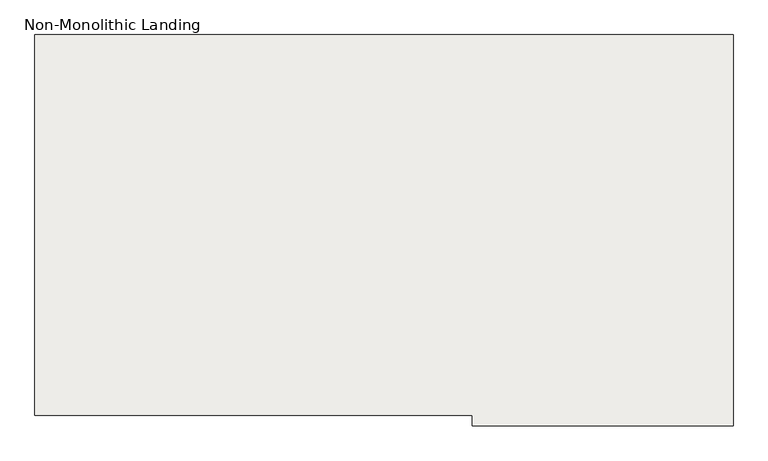
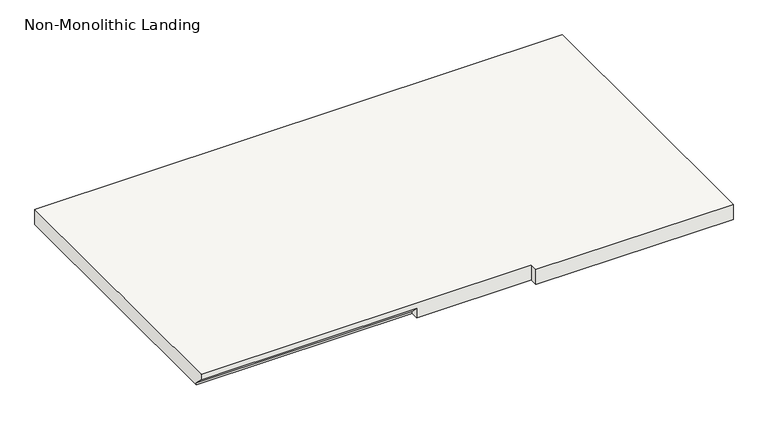
"""IFC4 building model written with IfcOpenShell, lengths in millimetres: slab geometry, Non-Monolithic Landing."""

from ifc_helpers import new_model, si_unit, origin, place, context, project, spatial, faceted_brep, source, transform, mapped, element, save


def non_monolithic_landing_d6ac0f27(model_context):
    return source(origin(), model_context, "Body", "Brep", [
        faceted_brep([(-10219.7292802, 8851.0516835, 1166.2833333), (-10219.7292802, 8876.4516835, 1140.8833333), (-9533.9292802, 8876.4516835, 1140.8833333), (-9533.9292802, 8851.0516835, 1166.2833333), (-9169.9689718, 8851.0516835, 1185.3333333), (-9169.9689718, 8825.6516835, 1185.3333333), (-8543.3292802, 8825.6516835, 1185.3333333), (-8543.3292802, 8851.0516835, 1185.3333333), (-8543.3292802, 9765.4516835, 1185.3333333), (-10219.7292802, 9765.4516835, 1185.3333333), (-10219.7292802, 8851.0516835, 1185.3333333), (-9533.9292802, 8876.4516835, 1134.5333333), (-10219.7292802, 8876.4516835, 1134.5333333), (-10219.7292802, 9765.4516835, 1134.5333333), (-8543.3292802, 9765.4516835, 1134.5333333), (-8543.3292802, 8851.0516835, 1134.5333333), (-8543.3292802, 8825.6516835, 1134.5333333), (-9169.9689718, 8825.6516835, 1134.5333333), (-9169.9689718, 8851.0516835, 1134.5333333), (-9533.9292802, 8851.0516835, 1134.5333333)], [[[0, 1, 2, 3]], [[4, 5, 6, 7, 8, 9, 10]], [[11, 12, 13, 14, 15, 16, 17, 18, 19]], [[12, 11, 2, 1]], [[11, 19, 3, 2]], [[4, 10, 0, 3, 19, 18]], [[5, 4, 18, 17]], [[6, 5, 17, 16]], [[7, 6, 16, 15]], [[8, 7, 15, 14]], [[9, 8, 14, 13]], [[10, 9, 13, 12, 1, 0]]]),
    ])


if __name__ == "__main__":
    model = new_model("IFC4")
    model_context = context("Model", 3, world=origin())
    ifc_project = project(units=[si_unit("LENGTHUNIT", "METRE", prefix="MILLI")], contexts=[model_context])
    site = spatial("IfcSite", under=ifc_project)
    building = spatial("IfcBuilding", under=site)
    placement = place(None, origin())
    non_monolithic_landing_shape = non_monolithic_landing_d6ac0f27(model_context)
    element("IfcSlab", 1, ObjectType="Non-Monolithic Landing", at=placement, inside=building, context=model_context, shape_type="MappedRepresentation", body=[
        mapped(non_monolithic_landing_shape, transform((0.0, 0.0, 0.0), x_axis=(1.0, 0.0, 0.0), y_axis=(0.0, 1.0, 0.0), z_axis=(0.0, 0.0, 1.0))),
    ])
    save(model, "model.ifc")
